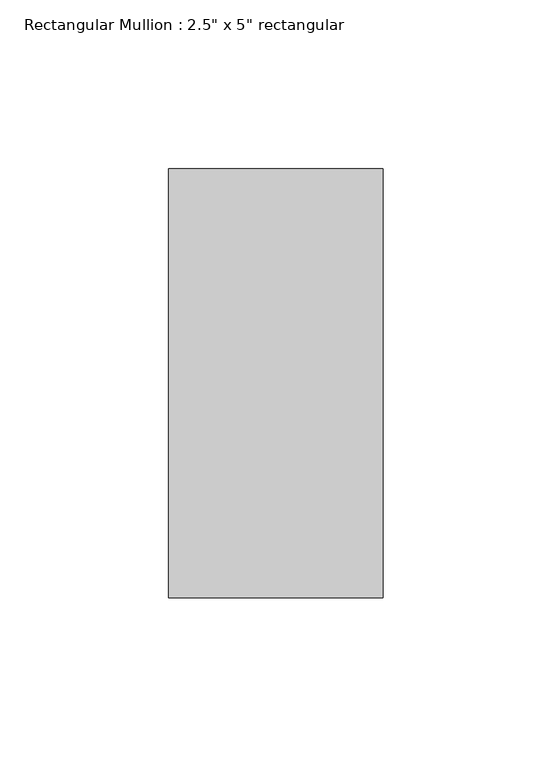
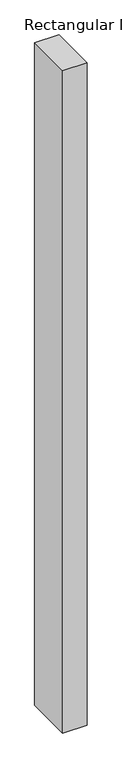
"""IFC4 building model written with IfcOpenShell, lengths in millimetres: member geometry."""

from ifc_helpers import new_model, si_unit, frame, origin, place, context, project, spatial, polyline, outline, extrude, source, transform, mapped, element, save


def member_2fae0574(model_context):
    return source(origin(), model_context, "Body", "SweptSolid", [
        extrude(outline(polyline([(0.0, 63.5), (0.0, -63.5), (-63.5, -63.5), (-63.5, 63.5), (0.0, 63.5)])), frame((0.0, 0.0, -1828.8), z_axis=(0.0, 0.0, 1.0), x_axis=(1.0, 0.0, 0.0)), (0.0, 0.0, 1.0), 1828.8),
    ])


if __name__ == "__main__":
    model = new_model("IFC4")
    model_context = context("Model", 3, world=origin())
    ifc_project = project(units=[si_unit("LENGTHUNIT", "METRE", prefix="MILLI")], contexts=[model_context])
    site = spatial("IfcSite", under=ifc_project)
    building = spatial("IfcBuilding", under=site)
    placement = place(None, origin())
    member_shape = member_2fae0574(model_context)
    element("IfcMember", 1, ObjectType="Rectangular Mullion : 2.5\" x 5\" rectangular", at=placement, inside=building, context=model_context, shape_type="MappedRepresentation", body=[
        mapped(member_shape, transform((0.0, 0.0, 0.0), x_axis=(1.0, 0.0, 0.0), y_axis=(0.0, 1.0, 0.0), z_axis=(0.0, 0.0, 1.0))),
    ])
    save(model, "model.ifc")

# Revit data of these elements
# Type "Rectangular Mullion : 2.5\" x 5\" rectangular"
#   built-in parameter 1007304 = 0.416667 (stored number, unit not read)
#   built-in parameter 1007301 = 0.104167 (stored number, unit not read)
#   built-in parameter 1007300 = 0.104167 (stored number, unit not read)
# Element 1 (IfcMember, "Rectangular Mullion : 2.5\" x 5\" rectangular")
#   Materials on its faces: "Aluminum"
# Materials
#   "Aluminum": class "Metal", colour RGB 247 247 247, transparency 0, Description = "Aluminum 6061", Cost = 0
